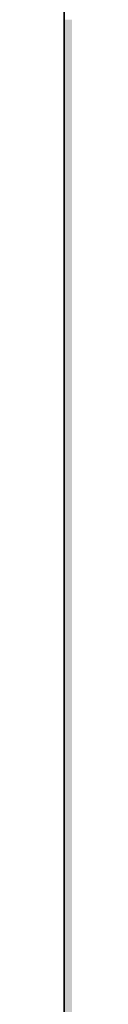
# Model space of a CAD drawing. Units: inches. Extents: x 2091 to 2899, y 967 to 2217.
# Tile 113 of 256: x 2203 to 2203, y 1131 to 1152. Entities that reach past the tile are written whole.
import ezdxf

# ---------------------------------------------------------------- set-up
doc = ezdxf.new("R2010")
doc.units = ezdxf.units.IN
doc.layers.add('A-WALL-PATT', color=141, linetype='Continuous', lineweight=13, true_color=0xadddf7)
doc.layers.add('C-PROP', color=7, linetype='Continuous', lineweight=35)

msp = doc.modelspace()

# ---------------------------------------------------------------- hatches: boundary and pattern name
at = {"layer": 'A-WALL-PATT'}
h = msp.add_hatch(color=256, dxfattribs=at)
h.dxf.hatch_style = 1
h.paths.add_polyline_path([(2212.144, 1941.419), (2387.644, 1941.419), (2387.644, 1824.419), (2392.144, 1824.419), (2392.144, 1941.419), (2609.644, 1941.419), (2609.644, 1825.919), (2614.144, 1825.919), (2614.144, 1941.419), (2794.144, 1941.419), (2794.144, 1928.762), (2803.144, 1928.762), (2803.144, 2050.919), (2203.144, 2050.919), (2203.144, 1900.758), (2212.144, 1900.758)])
h.paths.add_polyline_path([(2212.144, 1945.919), (2212.144, 2041.919), (2794.144, 2041.919), (2794.144, 1945.919), (2402.248, 1945.919), (2401.102, 1945.776), (2398.702, 1945.776)], flags=16)
h.paths.add_polyline_path([(2230.23, 1948.063), (2227.35, 1949.503), (2225.91, 1951.903), (2223.99, 1952.863), (2223.03, 1955.263), (2222.07, 1959.583), (2222.07, 1963.423), (2223.03, 1965.663), (2223.99, 1965.343), (2225.586, 1963.861), (2226.912, 1964.957), (2226.949, 1965.939), (2227.778, 1966.952), (2228.2, 1968.879), (2230.71, 1964.863), (2233.59, 1966.303), (2233.607, 1966.332), (2233.773, 1964.938), (2234.634, 1963.676), (2235.03, 1963.903), (2236.282, 1965.572), (2235.99, 1962.943), (2237.955, 1957.54), (2238.39, 1957.903), (2239.216, 1960.306), (2238.655, 1966.385), (2238.693, 1966.438), (2238.841, 1967.5), (2238.78, 1967.687), (2238.881, 1967.787), (2238.667, 1966.252), (2239.216, 1960.306), (2238.39, 1957.903), (2236.95, 1956.703), (2234.55, 1949.983)], flags=0)
h.paths.add_polyline_path([(2278.012, 1948.063), (2276.496, 1947.873), (2275.85, 1947.689), (2274.652, 1947.103)], flags=0)
h.paths.add_polyline_path([(2269.852, 1955.743), (2268.276, 1956.629), (2270.867, 1956.348), (2269.372, 1958.143), (2268.715, 1959.192), (2270.57, 1958.729), (2268.581, 1961.906), (2270.812, 1960.892), (2270.812, 1963.423), (2271.393, 1964.779), (2270.292, 1966.156), (2271.772, 1965.663), (2272.141, 1966.525), (2273.93, 1965.929), (2275.63, 1968.054), (2276.332, 1966.722), (2276.52, 1966.952), (2276.942, 1968.879), (2277.734, 1967.611), (2278.14, 1969.465), (2279.659, 1967.034), (2280.412, 1966.783), (2280.949, 1967.589), (2281.61, 1967.369), (2282.133, 1968.154), (2282.349, 1966.333), (2282.35, 1966.333), (2283.408, 1968.095), (2283.713, 1965.524), (2284.32, 1964.634), (2284.512, 1964.889), (2284.235, 1965.705), (2284.5, 1967.319), (2284.908, 1965.417), (2285.396, 1966.069), (2285.433, 1966.291), (2285.473, 1966.171), (2286.354, 1967.345), (2286.222, 1966.158), (2287.663, 1968.08), (2287.714, 1968.443), (2288.482, 1969.017), (2288.574, 1968.729), (2288.917, 1969.069), (2288.607, 1966.838), (2288.929, 1963.351), (2288.935, 1963.357), (2288.93, 1963.34), (2289.015, 1962.414), (2290.111, 1963.875), (2290.133, 1963.943), (2290.218, 1964.017), (2290.111, 1963.875), (2289.156, 1960.892), (2288.594, 1959.257), (2288.572, 1959.103), (2289.532, 1960.543), (2290.012, 1962.463), (2290.192, 1962.643), (2289.77, 1959.689), (2286.89, 1957.289), (2284.49, 1950.569), (2283.315, 1950.046), (2283.292, 1949.983), (2280.29, 1948.649), (2281.13, 1948.649), (2282.57, 1948.169), (2283.205, 1948.063), (2278.972, 1948.063), (2276.092, 1949.503), (2274.652, 1951.903), (2272.732, 1952.863)], flags=0)
h.paths.add_polyline_path([(2271.159, 1958.022), (2272.97, 1955.849), (2272.01, 1960.169), (2272.01, 1964.009), (2272.624, 1965.443), (2274.328, 1963.861), (2275.654, 1964.957), (2275.638, 1964.539), (2277.412, 1966.007), (2277.033, 1965.157), (2276.83, 1964.976), (2276.766, 1963.295), (2277.45, 1962.66), (2279.452, 1964.863), (2282.332, 1966.303), (2283.53, 1966.889), (2283.295, 1966.771), (2283.913, 1963.885), (2284.899, 1964.448), (2284.732, 1962.943), (2286.697, 1957.54), (2287.132, 1957.903), (2287.542, 1959.095), (2287.779, 1958.442), (2285.683, 1956.695), (2285.877, 1959.795), (2284.732, 1962.943), (2284.899, 1964.448), (2283.913, 1963.885), (2284.224, 1962.434), (2283.424, 1963.605), (2281.61, 1962.569), (2281.13, 1960.169), (2282.09, 1956.329), (2283.05, 1952.969), (2282.57, 1950.569), (2280.17, 1948.649), (2279.883, 1948.792), (2278.972, 1948.063), (2278.972, 1949.023), (2278.672, 1949.397), (2277.29, 1950.089), (2275.85, 1952.489), (2273.93, 1953.449), (2272.49, 1954.889), (2271.922, 1954.889), (2271.772, 1955.263)], flags=0)
h.paths.add_polyline_path([(2311.994, 1955.743), (2312.063, 1955.674), (2312.055, 1955.709)], flags=0)
h.paths.add_polyline_path([(2331.956, 1963.952), (2333.396, 1965.392), (2331.077, 1963.357), (2330.999, 1963.112)], flags=0)
h.paths.add_polyline_path([(2310.554, 1954.303), (2307.04, 1956.28), (2310.763, 1955.876), (2312.474, 1953.823), (2313.434, 1951.423), (2315.354, 1950.463), (2316.794, 1948.063), (2317.466, 1947.727), (2319.369, 1947.965), (2317.754, 1949.983), (2317.57, 1950.61), (2316.794, 1951.903), (2314.874, 1952.863), (2313.914, 1955.263), (2311.514, 1958.143), (2309.375, 1961.559), (2311.514, 1960.337), (2311.514, 1961.983), (2310.605, 1963.12), (2311.727, 1962.479), (2312.418, 1964.093), (2312.256, 1964.296), (2313.194, 1963.983), (2313.914, 1965.663), (2314.647, 1965.419), (2315.354, 1966.303), (2316.794, 1967.743), (2316.157, 1966.947), (2317.034, 1965.282), (2317.223, 1965.512), (2317.777, 1968.046), (2318.474, 1966.722), (2318.663, 1966.952), (2319.084, 1968.879), (2321.207, 1965.482), (2322.161, 1966.914), (2322.554, 1966.783), (2322.786, 1967.131), (2322.882, 1966.324), (2323.312, 1965.722), (2323.651, 1965.891), (2324.396, 1967.133), (2324.657, 1964.938), (2324.972, 1964.477), (2325.387, 1967.001), (2325.941, 1964.418), (2327.229, 1966.136), (2327.166, 1965.572), (2328.059, 1966.763), (2328.225, 1966.247), (2329.668, 1967.677), (2329.665, 1967.687), (2329.765, 1967.787), (2329.551, 1966.252), (2330.1, 1960.306), (2329.333, 1958.073), (2329.313, 1957.935), (2329.634, 1958.203), (2330.234, 1959.103), (2330.714, 1961.023), (2331.034, 1961.343), (2330.714, 1959.103), (2329.634, 1958.203), (2329.274, 1957.663), (2327.712, 1956.361), (2325.434, 1949.983), (2324.334, 1949.494), (2323.994, 1948.543), (2319.674, 1946.623), (2316.794, 1948.063), (2315.354, 1950.463), (2313.434, 1951.423)], flags=0)
h.paths.add_polyline_path([(2321.336, 1947.952), (2321.114, 1948.063), (2321.114, 1949.023), (2319.194, 1951.423), (2316.794, 1959.583), (2316.663, 1959.583), (2315.354, 1958.143), (2314.394, 1958.143), (2313.148, 1958.709), (2312.954, 1959.583), (2312.954, 1960.892), (2315.834, 1959.583), (2316.663, 1959.583), (2317.315, 1960.299), (2315.03, 1962.421), (2316.356, 1963.517), (2316.372, 1963.952), (2316.47, 1963.861), (2317.796, 1964.957), (2317.755, 1963.89), (2319.175, 1965.157), (2319.498, 1965.881), (2321.114, 1965.343), (2323.236, 1962.372), (2325.686, 1963.773), (2325.543, 1962.481), (2325.199, 1963.494), (2324.479, 1963.082), (2324.926, 1960.994), (2324.078, 1962.236), (2322.415, 1961.286), (2322.074, 1959.583), (2323.034, 1955.743), (2323.994, 1952.383), (2323.514, 1949.983), (2322.143, 1948.886), (2322.074, 1948.543)], flags=0)
h.paths.add_polyline_path([(2320.207, 1963.337), (2320.154, 1963.423), (2320.394, 1963.543)], flags=0)
h.paths.add_polyline_path([(2353.851, 1965.811), (2354.031, 1965.751), (2354.331, 1966.451), (2354.331, 1966.931)], flags=0)
h.paths.add_polyline_path([(2359.021, 1969.026), (2359.098, 1968.902), (2359.234, 1969.52), (2359.234, 1970)], flags=0)
h.paths.add_polyline_path([(2358.257, 1966.682), (2357.984, 1966.348), (2358.211, 1966.146), (2358.41, 1966.39)], flags=0)
h.paths.add_polyline_path([(2357.768, 1966.059), (2357.732, 1965.105), (2357.751, 1965.121), (2357.77, 1965.607), (2357.77, 1966.058)], flags=0)
h.paths.add_polyline_path([(2359.112, 1965.305), (2359.112, 1964.825), (2359.845, 1966.468), (2359.845, 1966.948)], flags=0)
h.paths.add_polyline_path([(2360.224, 1966.621), (2360.699, 1969.363), (2360.699, 1969.843), (2360.211, 1967.026), (2360.211, 1966.643)], flags=0)
h.paths.add_polyline_path([(2363.451, 1967.891), (2363.451, 1968.371), (2362.491, 1966.931), (2362.656, 1966.699)], flags=0)
h.paths.add_polyline_path([(2364.476, 1966.079), (2365.851, 1968.371), (2365.851, 1968.851), (2364.428, 1966.48)], flags=0)
h.paths.add_polyline_path([(2366.314, 1965.853), (2366.367, 1965.696), (2366.803, 1968.346), (2366.803, 1968.826)], flags=0)
h.paths.add_polyline_path([(2367.165, 1965.804), (2367.291, 1966.931), (2367.291, 1967.411), (2367.103, 1965.72)], flags=0)
h.paths.add_polyline_path([(2370.037, 1959.974), (2371.014, 1963.025), (2371.014, 1963.505), (2370.037, 1960.454)], flags=0)
h.paths.add_polyline_path([(2371.611, 1960.211), (2372.571, 1961.651), (2372.571, 1962.131), (2371.803, 1960.979)], flags=0)
h.paths.add_polyline_path([(2350.874, 1956.005), (2351.931, 1955.891), (2354.491, 1953.331), (2353.851, 1954.931), (2351.451, 1957.811), (2347.936, 1963.426), (2347.936, 1963.906), (2351.451, 1958.291), (2353.705, 1955.585), (2352.891, 1959.251), (2352.891, 1959.731), (2352.891, 1961.925), (2356.731, 1959.731), (2358.454, 1961.627), (2354.811, 1965.011), (2355.031, 1965.286), (2358.691, 1961.887), (2361.531, 1965.011), (2364.376, 1966.433), (2364.524, 1965.187), (2365.454, 1963.824), (2365.881, 1964.068), (2365.371, 1966.451), (2365.371, 1966.931), (2366.811, 1960.211), (2366.811, 1959.731), (2366.389, 1952.981), (2367.771, 1956.851), (2368.641, 1957.576), (2366.811, 1962.611), (2366.811, 1963.091), (2368.775, 1957.688), (2369.211, 1958.051), (2370.002, 1960.352), (2369.475, 1966.053), (2369.513, 1966.106), (2369.514, 1966.111), (2369.475, 1966.533), (2369.513, 1966.586), (2369.615, 1967.313), (2369.183, 1968.659), (2369.183, 1969.139), (2369.601, 1967.835), (2369.701, 1967.934), (2369.718, 1968.055), (2370.145, 1968.374), (2369.779, 1968.011), (2369.701, 1967.454), (2370.468, 1968.214), (2369.675, 1967.266), (2369.514, 1966.111), (2370.037, 1960.454), (2370.037, 1959.974), (2369.442, 1958.243), (2370.651, 1959.251), (2371.046, 1962.018), (2371.131, 1962.131), (2370.651, 1958.771), (2367.771, 1956.371), (2365.371, 1949.651), (2362.079, 1948.188), (2363.451, 1947.731), (2361.051, 1947.731), (2360.091, 1947.731), (2357.104, 1947.357), (2360.091, 1948.211), (2358.171, 1949.171), (2356.731, 1951.571), (2354.811, 1952.531), (2351.931, 1955.411)], flags=0)
h.paths.add_polyline_path([(2361.051, 1948.691), (2359.131, 1951.091), (2356.731, 1959.251), (2355.771, 1959.251), (2352.891, 1960.56), (2352.891, 1961.445), (2355.891, 1959.731), (2356.731, 1959.731), (2356.837, 1959.368), (2361.531, 1964.531), (2363.248, 1965.389), (2364.925, 1963.042), (2362.491, 1961.651), (2362.064, 1959.517), (2362.971, 1955.891), (2363.931, 1952.531), (2363.931, 1952.051), (2363.451, 1949.651), (2361.051, 1947.731)], flags=0)
h.paths.add_polyline_path([(2359.131, 1951.571), (2359.291, 1951.371), (2361.051, 1954.451), (2361.051, 1954.931)], flags=0)
h.paths.add_polyline_path([(2357.22, 1966.546), (2356.793, 1968.815), (2356.793, 1969.295), (2357.22, 1967.026)], flags=0)
h.paths.add_polyline_path([(2361.051, 1954.451), (2361.531, 1958.771), (2361.531, 1959.251), (2361.051, 1954.931)], flags=0)
h.paths.add_polyline_path([(2402.548, 1948.486), (2402.302, 1948.416), (2402.59, 1948.416)], flags=0)
h.paths.add_polyline_path([(2394.142, 1956.096), (2395.685, 1954.553), (2396.72, 1953.971), (2396.062, 1955.616), (2395.241, 1956.601), (2395.879, 1956.442), (2395.102, 1959.936), (2395.102, 1963.776), (2396.062, 1966.016), (2397.022, 1965.696), (2398.618, 1964.214), (2399.944, 1965.31), (2399.981, 1966.292), (2400.811, 1967.305), (2401.232, 1969.232), (2403.538, 1965.543), (2403.942, 1967.389), (2404.702, 1967.136), (2405.46, 1966.075), (2406.622, 1966.656), (2406.64, 1966.685), (2406.805, 1965.291), (2406.926, 1965.115), (2407.342, 1964.976), (2407.874, 1965.774), (2408.169, 1964.398), (2409.315, 1965.925), (2409.217, 1965.051), (2409.445, 1963.131), (2410.306, 1961.87), (2410.702, 1962.096), (2411.442, 1963.082), (2411.165, 1963.898), (2411.616, 1966.64), (2411.725, 1966.791), (2411.873, 1967.853), (2411.813, 1968.041), (2411.913, 1968.14), (2411.699, 1966.605), (2412.248, 1960.659), (2413.225, 1963.71), (2414.378, 1964.721), (2414.513, 1965.693), (2414.453, 1965.881), (2414.553, 1965.98), (2414.378, 1964.721), (2414.52, 1964.846), (2414.365, 1964.631), (2414.339, 1964.445), (2414.888, 1958.499), (2414.062, 1956.096), (2412.622, 1954.896), (2410.171, 1948.033), (2410.017, 1948.084), (2405.902, 1946.256), (2405.902, 1947.216), (2405.204, 1948.089), (2404.222, 1948.416), (2403.262, 1948.416), (2400.382, 1949.856), (2399.662, 1951.056), (2397.982, 1952.736), (2397.022, 1953.216), (2395.685, 1954.553), (2392.657, 1956.257)], flags=0)
h.paths.add_polyline_path([(2409.086, 1964.407), (2409.13, 1964.276), (2409.262, 1964.496)], flags=0)
h.paths.add_polyline_path([(2397.742, 1961.616), (2398.702, 1963.856), (2399.662, 1963.536), (2401.427, 1965.741), (2401.791, 1966.559), (2402.071, 1965.071), (2402.836, 1964.393), (2403.262, 1964.915), (2403.338, 1964.771), (2402.616, 1963.976), (2402.499, 1960.902), (2403.543, 1959.932), (2404.413, 1960.89), (2404.702, 1962.336), (2407.916, 1964.172), (2409.52, 1961.927), (2410.987, 1957.893), (2411.422, 1958.256), (2412.048, 1960.076), (2412.41, 1959.079), (2411.676, 1958.467), (2411.662, 1958.256), (2411.626, 1958.426), (2409.982, 1957.056), (2407.582, 1950.336), (2403.262, 1948.416), (2403.262, 1949.376), (2401.342, 1951.776), (2399.417, 1958.324), (2397.742, 1959.085), (2397.742, 1959.97), (2397.102, 1960.336), (2397.742, 1960.045)], flags=0)
h.paths.add_polyline_path([(2405.902, 1952.976), (2405.95, 1953.408), (2406.017, 1953.176)], flags=0)
h.paths.add_polyline_path([(2449.818, 1967.114), (2449.752, 1967.136), (2449.794, 1967.078)], flags=0)
h.paths.add_polyline_path([(2451.698, 1966.618), (2451.741, 1966.69), (2451.692, 1966.666)], flags=0)
h.paths.add_polyline_path([(2454.344, 1965.738), (2455.752, 1967.616), (2455.992, 1968.096), (2454.364, 1965.925)], flags=0)
h.paths.add_polyline_path([(2457.547, 1968.864), (2457.787, 1969.344), (2457.054, 1968.796), (2457.008, 1968.46)], flags=0)
h.paths.add_polyline_path([(2456.922, 1967.857), (2456.802, 1968.229), (2456.723, 1967.66)], flags=0)
h.paths.add_polyline_path([(2457.302, 1967.377), (2457.542, 1967.857), (2456.81, 1966.84), (2456.741, 1966.7), (2456.749, 1966.608)], flags=0)
h.paths.add_polyline_path([(2458.275, 1963.71), (2458.155, 1963.335), (2460.354, 1965.265), (2460.594, 1965.745)], flags=0)
h.paths.add_polyline_path([(2458.392, 1962.816), (2458.364, 1962.618), (2459.592, 1964.256), (2459.832, 1964.736)], flags=0)
h.paths.add_polyline_path([(2459.352, 1962.816), (2459.272, 1962.496), (2460.072, 1963.296), (2460.312, 1963.776)], flags=0)
h.paths.add_polyline_path([(2458.68, 1960.608), (2458.632, 1960.416), (2459.592, 1961.856), (2459.832, 1962.336)], flags=0)
h.paths.add_polyline_path([(2437.838, 1956.243), (2439.192, 1956.096), (2441.352, 1953.936), (2440.872, 1955.136), (2438.472, 1958.016), (2438.072, 1958.656), (2438.712, 1958.496), (2440.64, 1956.183), (2439.912, 1959.456), (2439.912, 1963.296), (2441.352, 1966.656), (2441.592, 1967.136), (2441.112, 1966.016), (2442.072, 1965.696), (2443.989, 1968.092), (2444.241, 1966.751), (2444.917, 1966.152), (2445.677, 1967.08), (2446.255, 1969.725), (2446.495, 1970.205), (2446.282, 1969.232), (2447.363, 1967.503), (2447.72, 1969.568), (2447.96, 1970.048), (2447.485, 1967.307), (2448.792, 1965.216), (2448.472, 1964.864), (2448.552, 1964.736), (2451.452, 1966.186), (2451.615, 1964.811), (2452.308, 1963.796), (2453.235, 1964.326), (2454.072, 1960.416), (2453.629, 1953.318), (2454.792, 1956.576), (2455.032, 1957.056), (2455.719, 1957.628), (2453.832, 1962.816), (2453.941, 1963.794), (2453.335, 1965.578), (2453.824, 1968.551), (2454.064, 1969.031), (2453.575, 1966.058), (2454.04, 1964.688), (2453.832, 1962.816), (2455.719, 1957.628), (2456.367, 1958.168), (2457.058, 1960.179), (2457.298, 1960.659), (2456.472, 1958.256), (2457.718, 1959.294), (2457.672, 1958.976), (2454.89, 1956.657), (2453.614, 1953.085), (2453.592, 1952.736), (2453.352, 1952.256), (2453.36, 1952.372), (2452.632, 1950.336), (2452.392, 1949.856), (2449.204, 1948.439), (2450.712, 1947.936), (2448.072, 1947.936), (2447.112, 1947.936), (2444.552, 1947.616), (2447.2, 1948.372), (2445.192, 1949.376), (2443.752, 1951.776), (2441.832, 1952.736), (2438.952, 1955.616)], flags=0)
h.paths.add_polyline_path([(2443.992, 1959.936), (2444.04, 1959.773), (2444.122, 1959.862)], flags=0)
h.paths.add_polyline_path([(2442.912, 1959.936), (2443.032, 1959.936), (2442.446, 1960.202)], flags=0)
h.paths.add_polyline_path([(2444.983, 1965.02), (2445.279, 1965.265), (2445.519, 1965.745), (2444.994, 1965.31)], flags=0)
h.paths.add_polyline_path([(2446.133, 1965.03), (2446.33, 1965.471), (2444.97, 1964.258), (2444.73, 1963.778)], flags=0)
h.paths.add_polyline_path([(2442.792, 1959.456), (2443.752, 1959.456), (2446.152, 1951.296), (2446.412, 1951.751), (2446.392, 1951.776), (2448.081, 1954.73), (2448.552, 1958.976), (2441.832, 1965.216), (2442.155, 1965.619), (2448.792, 1959.456), (2448.312, 1955.136), (2448.072, 1954.656), (2446.412, 1951.751), (2448.312, 1949.376), (2448.312, 1948.416), (2450.541, 1950.199), (2450.952, 1952.256), (2449.992, 1955.616), (2449.032, 1959.456), (2449.512, 1961.856), (2449.752, 1962.336), (2449.675, 1961.949), (2452.995, 1963.846), (2453.064, 1963.519), (2452.885, 1963.783), (2449.675, 1961.949), (2449.272, 1959.936), (2450.232, 1956.096), (2451.192, 1952.736), (2450.712, 1950.336), (2450.472, 1949.856), (2448.072, 1947.936), (2448.072, 1948.536), (2445.432, 1949.856), (2443.992, 1952.256), (2442.072, 1953.216), (2441.112, 1955.616), (2440.152, 1959.936), (2440.152, 1960.656)], flags=0)
h.paths.add_polyline_path([(2456.692, 1966.986), (2457.608, 1968.081), (2457.848, 1968.561), (2456.932, 1967.466)], flags=0)
h.paths.add_polyline_path([(2489.897, 1966.58), (2489.943, 1966.189), (2490.747, 1967.53), (2491.319, 1968.951)], flags=0)
h.paths.add_polyline_path([(2473.562, 1956.407), (2477.14, 1956.019), (2476.955, 1956.241), (2475.108, 1957.28), (2476.347, 1956.97), (2475.187, 1958.824), (2476.919, 1958.391), (2475.412, 1960.799), (2477.787, 1959.719), (2477.787, 1962.25), (2477.637, 1962.438), (2477.823, 1962.332), (2478.359, 1963.584), (2478.359, 1963.671), (2477.324, 1964.965), (2478.715, 1964.501), (2479.319, 1965.911), (2480.279, 1965.591), (2481.784, 1967.472), (2482.116, 1965.705), (2482.881, 1965.028), (2483.209, 1965.429), (2483.22, 1965.715), (2483.076, 1965.989), (2483.712, 1966.766), (2484.13, 1968.679), (2484.702, 1970.1), (2484.489, 1969.127), (2486.503, 1965.905), (2487.387, 1965.61), (2488.153, 1966.759), (2488.717, 1965.97), (2489.2, 1966.212), (2489.331, 1965.111), (2490.394, 1963.622), (2490.661, 1963.775), (2490.494, 1964.554), (2490.923, 1963.925), (2491.319, 1964.151), (2491.333, 1964.17), (2491.21, 1964.532), (2491.282, 1964.966), (2491.426, 1964.293), (2494.076, 1967.828), (2494.498, 1966.515), (2494.598, 1966.614), (2494.689, 1967.27), (2495.107, 1967.582), (2495.13, 1967.748), (2495.07, 1967.936), (2495.17, 1968.035), (2495.032, 1967.044), (2495.754, 1967.759), (2494.982, 1966.686), (2494.956, 1966.5), (2495.479, 1960.837), (2495.91, 1962.184), (2496.482, 1963.605), (2496.073, 1962.327), (2496.769, 1962.938), (2496.599, 1962.711), (2496.119, 1959.351), (2496.733, 1960.272), (2496.987, 1961.29), (2497.559, 1962.711), (2497.079, 1960.791), (2496.507, 1959.37), (2495.547, 1957.93), (2492.759, 1955.606), (2490.839, 1950.231), (2490.267, 1948.81), (2485.947, 1946.89), (2483.067, 1948.33), (2481.627, 1950.73), (2479.707, 1951.69), (2476.827, 1954.57)], flags=0)
h.paths.add_polyline_path([(2485.577, 1948.313), (2485.559, 1948.311), (2485.579, 1948.311)], flags=0)
h.paths.add_polyline_path([(2478.645, 1954.551), (2478.109, 1956.963), (2479.319, 1955.511), (2480.279, 1953.111), (2482.199, 1952.151), (2483.639, 1949.751), (2486.519, 1948.311), (2486.519, 1949.271), (2484.739, 1951.496), (2484.027, 1950.25), (2481.627, 1958.41), (2482.375, 1959.233), (2482.199, 1959.831), (2483.198, 1960.929), (2479.707, 1964.17), (2480.603, 1965.29), (2481.875, 1964.109), (2482.666, 1964.764), (2482.615, 1963.422), (2482.989, 1963.075), (2484.008, 1963.984), (2484.684, 1965.498), (2484.58, 1965.405), (2485.357, 1967.147), (2485.121, 1965.781), (2486.427, 1963.69), (2488.145, 1964.549), (2489.822, 1962.202), (2490.747, 1962.73), (2492, 1964.4), (2492.076, 1965.087), (2492.213, 1964.684), (2492.485, 1965.047), (2492.279, 1963.191), (2494.244, 1957.788), (2494.563, 1958.054), (2494.933, 1959.133), (2495.505, 1960.554), (2494.679, 1958.151), (2494.107, 1956.73), (2494.563, 1958.054), (2493.409, 1957.092), (2491.707, 1961.77), (2492, 1964.4), (2490.747, 1962.73), (2487.712, 1960.996), (2487.479, 1959.831), (2488.439, 1955.991), (2489.399, 1952.631), (2488.919, 1950.231), (2488.577, 1949.957), (2488.347, 1948.81), (2487.652, 1948.254), (2487.479, 1948.311), (2486.519, 1948.311), (2483.639, 1949.751), (2482.199, 1952.151), (2480.279, 1953.111), (2478.839, 1954.551)], flags=0)
h.paths.add_polyline_path([(2526.648, 1966.988), (2526.517, 1967.031), (2526.6, 1966.915)], flags=0)
h.paths.add_polyline_path([(2528.471, 1966.447), (2528.574, 1966.62), (2528.457, 1966.561)], flags=0)
h.paths.add_polyline_path([(2534.133, 1967.496), (2534.157, 1967.543), (2534.06, 1967.408)], flags=0)
h.paths.add_polyline_path([(2536.162, 1964.051), (2535.157, 1962.711), (2535.101, 1962.316), (2536.117, 1963.671), (2536.421, 1964.278)], flags=0)
h.paths.add_polyline_path([(2535.157, 1959.831), (2536.117, 1961.271), (2536.597, 1962.231), (2535.253, 1960.215)], flags=0)
h.paths.add_polyline_path([(2513.249, 1956.285), (2516.221, 1955.963), (2514.997, 1957.431), (2514.196, 1958.712), (2515.477, 1958.391), (2516.932, 1956.646), (2516.437, 1958.871), (2516.437, 1962.711), (2516.873, 1963.727), (2515.346, 1965.635), (2517.397, 1964.951), (2517.877, 1966.071), (2518.357, 1967.031), (2517.877, 1965.911), (2518.837, 1965.591), (2520.487, 1967.653), (2520.766, 1966.166), (2521.53, 1965.489), (2521.781, 1965.795), (2521.801, 1966.307), (2521.478, 1966.921), (2521.246, 1967.126), (2521.178, 1967.491), (2521.478, 1966.921), (2522.01, 1966.449), (2522.257, 1966.75), (2522.78, 1969.14), (2523.26, 1970.1), (2523.047, 1969.127), (2524.673, 1966.526), (2526.037, 1966.071), (2526.795, 1965.01), (2527.977, 1965.601), (2528.14, 1964.227), (2528.665, 1963.458), (2529.389, 1963.872), (2529.33, 1964.147), (2529.481, 1963.925), (2529.877, 1964.151), (2529.984, 1964.293), (2529.789, 1965.203), (2530.062, 1964.398), (2532.802, 1968.051), (2533.148, 1966.976), (2533.248, 1967.075), (2533.339, 1967.731), (2533.673, 1967.98), (2533.728, 1968.035), (2533.514, 1966.5), (2534.025, 1960.972), (2534.56, 1962.645), (2535.04, 1963.605), (2534.063, 1960.554), (2533.237, 1958.151), (2534.288, 1959.027), (2534.197, 1958.391), (2531.513, 1956.154), (2529.397, 1950.231), (2528.917, 1949.271), (2526.449, 1948.174), (2527.477, 1947.831), (2530.357, 1947.351), (2524.597, 1947.351), (2521.717, 1948.791), (2520.277, 1951.191), (2518.357, 1952.151), (2515.477, 1955.031)], flags=0)
h.paths.add_polyline_path([(2523.935, 1967.19), (2523.62, 1966.484), (2523.77, 1966.242)], flags=0)
h.paths.add_polyline_path([(2518.837, 1953.111), (2517.877, 1955.511), (2516.885, 1959.977), (2516.917, 1959.962), (2516.917, 1962.025), (2520.757, 1959.831), (2522.025, 1961.226), (2518.357, 1964.631), (2519.003, 1965.438), (2520.433, 1964.109), (2521.301, 1964.827), (2521.245, 1963.355), (2525.638, 1959.276), (2526.037, 1961.271), (2529.397, 1963.191), (2530.65, 1964.861), (2530.665, 1964.998), (2530.692, 1964.917), (2531.088, 1965.445), (2530.946, 1964.169), (2530.692, 1964.917), (2529.397, 1963.191), (2526.363, 1961.457), (2526.037, 1959.831), (2526.997, 1955.991), (2527.957, 1952.631), (2527.477, 1950.231), (2527.134, 1949.957), (2526.974, 1949.154), (2526.697, 1949.031), (2524.597, 1947.351), (2524.597, 1948.311), (2524.277, 1948.711), (2522.197, 1949.751), (2520.757, 1952.151)], flags=0)
h.paths.add_polyline_path([(2520.277, 1958.871), (2520.853, 1959.505), (2523.157, 1951.671), (2524.614, 1954.22), (2524.597, 1954.071), (2522.677, 1950.711)], flags=0)
h.paths.add_polyline_path([(2559.371, 1966.311), (2559.398, 1966.325), (2559.402, 1966.345)], flags=0)
h.paths.add_polyline_path([(2549.771, 1957.191), (2552.651, 1954.311), (2552.134, 1955.603), (2550.611, 1957.431), (2547.096, 1963.046), (2545.776, 1965.206), (2549.291, 1959.591), (2551.691, 1956.711), (2550.793, 1960.752), (2550.731, 1960.78), (2550.731, 1964.871), (2551.691, 1967.111), (2552.651, 1966.791), (2554.247, 1965.309), (2555.034, 1965.96), (2555.582, 1966.645), (2555.61, 1967.387), (2556.439, 1968.401), (2556.861, 1970.327), (2559.371, 1966.311), (2560.691, 1964.151), (2562.409, 1965.01), (2561.651, 1966.071), (2560.331, 1968.231), (2561.758, 1966.233), (2562.347, 1967.116), (2562.434, 1966.387), (2563.128, 1965.37), (2563.571, 1965.591), (2563.588, 1965.62), (2563.363, 1967.524), (2563.722, 1965.844), (2565.06, 1968.073), (2564.733, 1965.129), (2565.118, 1963.333), (2567.445, 1966.436), (2567.316, 1967.833), (2567.354, 1967.886), (2567.502, 1968.948), (2567.441, 1969.136), (2567.542, 1969.235), (2567.328, 1967.7), (2567.877, 1961.754), (2568.747, 1964.47), (2568.636, 1965.673), (2568.674, 1965.726), (2568.822, 1966.788), (2568.761, 1966.976), (2568.862, 1967.075), (2568.648, 1965.54), (2568.726, 1964.693), (2568.854, 1964.805), (2568.747, 1964.47), (2568.817, 1963.706), (2568.971, 1963.911), (2568.866, 1963.177), (2569.197, 1959.594), (2568.371, 1957.191), (2566.931, 1955.991), (2564.62, 1949.521), (2564.651, 1949.511), (2564.617, 1949.511), (2564.531, 1949.271), (2560.211, 1947.351), (2557.331, 1948.791), (2556.045, 1950.934), (2556.011, 1950.951), (2555.857, 1951.208), (2553.971, 1952.151), (2551.091, 1955.031), (2546.65, 1957.53)], flags=0)
h.paths.add_polyline_path([(2567.026, 1959.33), (2567.035, 1959.305), (2567.051, 1959.351)], flags=0)
h.paths.add_polyline_path([(2551.968, 1962.518), (2553.011, 1964.951), (2553.971, 1964.631), (2555.567, 1963.149), (2556.893, 1964.246), (2556.93, 1965.227), (2557.144, 1965.489), (2556.42, 1966.131), (2556.391, 1966.105), (2556.38, 1966.166), (2556.42, 1966.131), (2556.952, 1966.605), (2557.092, 1966.919), (2557.571, 1966.01), (2557.759, 1966.241), (2557.418, 1964.68), (2556.893, 1964.246), (2556.807, 1961.998), (2560.691, 1958.391), (2560.636, 1957.893), (2560.811, 1957.191), (2561.771, 1953.831), (2561.291, 1951.431), (2559.11, 1949.687), (2559.156, 1949.629), (2563.027, 1951.349), (2562.611, 1949.271), (2560.211, 1947.351), (2560.211, 1948.311), (2559.251, 1949.511), (2558.891, 1949.511), (2558.891, 1949.961), (2558.291, 1950.711), (2558.054, 1951.518), (2556.971, 1952.871), (2555.068, 1959.341), (2552.051, 1961.065), (2552.051, 1962.471)], flags=0)
h.paths.add_polyline_path([(2588.33, 1958.391), (2588.61, 1958.111), (2588.553, 1958.367)], flags=0)
h.paths.add_polyline_path([(2594.745, 1950.493), (2593.958, 1953.172), (2593.13, 1954.551), (2591.21, 1955.511), (2590.25, 1957.911), (2588.309, 1960.24), (2586.177, 1961.209), (2587.85, 1960.791), (2587.253, 1961.744), (2588.441, 1961.065), (2588.441, 1962.656), (2588.422, 1962.665), (2588.441, 1962.711), (2586.914, 1964.62), (2588.877, 1963.728), (2589.29, 1964.692), (2589.29, 1966.071), (2590.25, 1968.311), (2591.21, 1967.991), (2592.806, 1966.509), (2594.132, 1967.606), (2594.169, 1968.587), (2594.999, 1969.601), (2595.42, 1971.527), (2597.93, 1967.511), (2600.81, 1968.951), (2600.827, 1968.98), (2600.993, 1967.587), (2601.854, 1966.325), (2602.107, 1966.47), (2602.236, 1967.255), (2602.357, 1966.693), (2603.502, 1968.221), (2603.21, 1965.591), (2605.175, 1960.188), (2605.507, 1960.465), (2605.026, 1965.673), (2605.064, 1965.726), (2605.212, 1966.788), (2605.152, 1966.976), (2605.252, 1967.075), (2605.343, 1967.731), (2605.953, 1968.187), (2605.875, 1969.033), (2605.913, 1969.086), (2606.061, 1970.148), (2606, 1970.336), (2606.101, 1970.435), (2605.887, 1968.9), (2606.436, 1962.954), (2605.61, 1960.551), (2605.997, 1960.874), (2606.564, 1962.645), (2608.241, 1964.117), (2608.01, 1963.191), (2607.05, 1961.751), (2606.631, 1961.402), (2606.201, 1958.391), (2603.321, 1955.991), (2600.921, 1949.271), (2596.601, 1947.351), (2593.721, 1948.791), (2592.857, 1950.231), (2592.65, 1950.231)], flags=0)
h.paths.add_polyline_path([(2596.601, 1947.351), (2596.601, 1948.311), (2594.681, 1950.711), (2596.155, 1953.29), (2595.53, 1954.071), (2593.199, 1961.996), (2592.651, 1962.505), (2591.78, 1963.003), (2593.283, 1964.246), (2593.32, 1965.227), (2594.15, 1966.241), (2594.571, 1968.167), (2596.183, 1965.589), (2596.951, 1966.435), (2598.041, 1966.071), (2598.799, 1965.01), (2599.961, 1965.591), (2599.979, 1965.62), (2600.144, 1964.227), (2601.005, 1962.965), (2601.401, 1963.191), (2602.653, 1964.861), (2602.361, 1962.231), (2603.793, 1958.295), (2601.978, 1953.212), (2601.946, 1952.709), (2599.469, 1951.608), (2599.001, 1949.271)], flags=0)
h.paths.add_polyline_path([(2597.561, 1958.871), (2597.671, 1959.419), (2597.595, 1958.736)], flags=0)
h.paths.add_polyline_path([(2623.666, 1961.254), (2625.519, 1960.791), (2624.966, 1961.676), (2627.199, 1960.66), (2627.199, 1961.151), (2626.959, 1962.231), (2626.959, 1963.491), (2625.582, 1965.212), (2626.959, 1964.425), (2626.959, 1965.831), (2626.869, 1965.861), (2627.919, 1968.311), (2628.879, 1967.991), (2630.475, 1966.509), (2631.801, 1967.606), (2631.838, 1968.587), (2632.668, 1969.601), (2633.089, 1971.527), (2635.599, 1967.511), (2638.479, 1968.951), (2638.497, 1968.98), (2638.662, 1967.587), (2639.176, 1966.833), (2639.78, 1967.84), (2640.026, 1966.693), (2641.171, 1968.221), (2640.879, 1965.591), (2641.114, 1964.945), (2641.411, 1965.341), (2641.308, 1964.412), (2642.844, 1960.188), (2643.279, 1960.551), (2644.085, 1962.895), (2643.784, 1966.153), (2643.807, 1966.185), (2643.601, 1968.418), (2643.523, 1968.661), (2643.73, 1970.148), (2643.67, 1970.336), (2643.77, 1970.435), (2643.556, 1968.9), (2643.601, 1968.418), (2643.91, 1967.456), (2644.01, 1967.555), (2643.812, 1966.132), (2644.105, 1962.954), (2644.239, 1961.351), (2644.719, 1961.751), (2645.033, 1962.222), (2645.322, 1963.125), (2646.076, 1963.787), (2645.033, 1962.222), (2644.345, 1960.074), (2643.519, 1957.671), (2642.079, 1956.471), (2639.72, 1949.864), (2639.876, 1949.838), (2635.359, 1947.831), (2632.479, 1949.271), (2631.039, 1951.671), (2629.119, 1952.631), (2628.159, 1955.031), (2625.759, 1957.911)], flags=0)
h.paths.add_polyline_path([(2627.816, 1956.574), (2627.374, 1958.566), (2626.376, 1959.763), (2627.199, 1959.351), (2627.374, 1958.566), (2627.919, 1957.911), (2628.879, 1955.511), (2630.799, 1954.551), (2632.239, 1952.151), (2633.315, 1951.613), (2631.039, 1959.351), (2631.498, 1959.856), (2630.799, 1962.231), (2631.45, 1962.947), (2630.715, 1963.629), (2632.041, 1964.726), (2632.078, 1965.707), (2632.292, 1965.969), (2631.705, 1966.489), (2633.136, 1967.766), (2633.329, 1968.647), (2634.675, 1966.494), (2635.208, 1967.081), (2636.799, 1966.551), (2637.676, 1967.867), (2638.994, 1966.022), (2639.705, 1966.429), (2641.119, 1959.831), (2640.93, 1956.806), (2639.439, 1952.631), (2638.227, 1952.093), (2637.759, 1949.751), (2635.359, 1947.831), (2635.359, 1948.791), (2633.439, 1951.191), (2633.315, 1951.613), (2632.239, 1952.151), (2630.799, 1954.551), (2628.879, 1955.511)], flags=0)
h.paths.add_polyline_path([(2637.759, 1953.831), (2637.279, 1955.511), (2636.319, 1959.351), (2636.799, 1961.751), (2639.234, 1963.142), (2637.557, 1965.49), (2638.739, 1966.081), (2638.902, 1964.707), (2639.763, 1963.445), (2636.799, 1961.751), (2636.532, 1960.418), (2637.039, 1958.391), (2637.999, 1955.031)], flags=0)
h.paths.add_polyline_path([(2668.567, 1951.431), (2667.607, 1953.831), (2665.207, 1956.711), (2662.294, 1961.365), (2665.447, 1959.591), (2666.647, 1958.391), (2666.647, 1959.975), (2666.058, 1960.682), (2666.647, 1960.345), (2666.647, 1961.991), (2666.7, 1962.114), (2666.407, 1963.431), (2666.407, 1967.271), (2667.367, 1969.511), (2668.327, 1969.191), (2669.923, 1967.709), (2671.249, 1968.806), (2671.286, 1969.787), (2672.116, 1970.801), (2672.537, 1972.727), (2675.047, 1968.711), (2677.927, 1970.151), (2677.945, 1970.18), (2678.11, 1968.787), (2678.971, 1967.525), (2679.367, 1967.751), (2680.62, 1969.421), (2680.327, 1966.791), (2682.292, 1961.388), (2682.727, 1961.751), (2683.358, 1963.587), (2683.232, 1964.953), (2683.27, 1965.006), (2683.393, 1965.889), (2683.36, 1966.249), (2683.358, 1966.256), (2683.359, 1966.257), (2682.992, 1970.233), (2683.03, 1970.286), (2683.178, 1971.348), (2683.118, 1971.536), (2683.218, 1971.635), (2683.004, 1970.1), (2683.359, 1966.257), (2683.458, 1966.355), (2683.393, 1965.889), (2683.414, 1965.665), (2684.424, 1966.872), (2683.553, 1964.154), (2683.358, 1963.587), (2683.793, 1958.874), (2682.967, 1956.471), (2681.527, 1955.271), (2680.109, 1951.3), (2680.085, 1950.912), (2679.977, 1950.93), (2679.127, 1948.551), (2674.807, 1946.631), (2671.927, 1948.071), (2670.487, 1950.471)], flags=0)
h.paths.add_polyline_path([(2671.936, 1953.227), (2671.687, 1953.351), (2670.247, 1955.751), (2668.327, 1956.711), (2667.357, 1959.138), (2669.527, 1958.151), (2670.487, 1958.151), (2671.479, 1959.242), (2670.684, 1961.945), (2668.89, 1963.612), (2667.307, 1964.331), (2668.567, 1963.911), (2668.831, 1964.241), (2670.247, 1963.431), (2672.422, 1965.823), (2672.777, 1967.447), (2673.234, 1966.716), (2674.412, 1968.012), (2673.981, 1965.522), (2675.287, 1963.431), (2675.554, 1963.564), (2675.932, 1965.456), (2676.247, 1965.351), (2677.005, 1964.29), (2678.167, 1964.871), (2679.607, 1967.271), (2680.327, 1963.911), (2680.307, 1963.577), (2680.347, 1963.458), (2680.86, 1964.141), (2680.567, 1961.511), (2681.104, 1960.037), (2678.887, 1953.831), (2677.092, 1953.033), (2677.687, 1950.951), (2677.207, 1948.551), (2674.807, 1946.631), (2674.807, 1947.591), (2672.887, 1949.991)], flags=0)
h.paths.add_polyline_path([(2673.985, 1951.911), (2674.567, 1952.931), (2674.567, 1951.911), (2676.967, 1953.831), (2677.447, 1956.231), (2676.487, 1959.591), (2676.247, 1960.551), (2679.73, 1962.541), (2680.059, 1961.002), (2679.211, 1962.245), (2676.247, 1960.551), (2676.487, 1959.591), (2677.447, 1956.231), (2676.967, 1953.831), (2674.567, 1951.911)], flags=0)
h.paths.add_polyline_path([(2707.479, 1952.815), (2706.519, 1955.215), (2705.559, 1959.535), (2705.559, 1963.375), (2706.519, 1965.615), (2707.479, 1965.295), (2709.075, 1963.813), (2710.401, 1964.909), (2710.438, 1965.891), (2711.268, 1966.904), (2711.689, 1968.831), (2714.199, 1964.815), (2717.079, 1966.255), (2717.097, 1966.284), (2717.262, 1964.89), (2718.123, 1963.628), (2718.519, 1963.855), (2719.771, 1965.524), (2719.479, 1962.895), (2721.444, 1957.492), (2721.879, 1957.855), (2722.705, 1960.258), (2722.144, 1966.337), (2722.182, 1966.39), (2722.33, 1967.452), (2722.27, 1967.639), (2722.37, 1967.739), (2722.156, 1966.204), (2722.705, 1960.258), (2721.879, 1957.855), (2720.439, 1956.655), (2718.039, 1949.935), (2713.719, 1948.015), (2710.839, 1949.455), (2709.399, 1951.855)], flags=0)
h.paths.add_polyline_path([(2749.301, 1952.815), (2748.341, 1955.215), (2747.381, 1959.535), (2747.381, 1963.375), (2748.341, 1965.615), (2749.301, 1965.295), (2750.897, 1963.813), (2752.223, 1964.909), (2752.26, 1965.891), (2753.09, 1966.904), (2753.511, 1968.831), (2756.021, 1964.815), (2758.901, 1966.255), (2758.919, 1966.284), (2759.084, 1964.89), (2759.945, 1963.628), (2760.341, 1963.855), (2761.593, 1965.524), (2761.301, 1962.895), (2763.266, 1957.492), (2763.701, 1957.855), (2764.527, 1960.258), (2763.966, 1966.337), (2764.004, 1966.39), (2764.152, 1967.452), (2764.092, 1967.639), (2764.192, 1967.739), (2763.978, 1966.204), (2764.527, 1960.258), (2763.701, 1957.855), (2762.261, 1956.655), (2759.861, 1949.935), (2755.541, 1948.015), (2752.661, 1949.455), (2751.221, 1951.855)], flags=0)
h.paths.add_polyline_path([(2212.144, 1819.935), (2203.144, 1819.935), (2203.144, 1739.98), (2212.144, 1739.98), (2212.144, 1780.919), (2392.144, 1780.919), (2392.144, 1783.919), (2212.144, 1783.919)])
h.paths.add_polyline_path([(2803.144, 1847.939), (2794.144, 1847.939), (2794.144, 1785.419), (2609.644, 1785.419), (2493.876, 1785.419), (2493.876, 1780.919), (2609.644, 1780.919), (2794.144, 1780.919), (2794.144, 1696.919), (2609.376, 1696.919), (2609.376, 1742.919), (2604.876, 1742.919), (2604.876, 1644.419), (2609.376, 1644.419), (2609.376, 1692.419), (2794.144, 1692.419), (2794.144, 1668.165), (2803.144, 1668.165)])
h.paths.add_polyline_path([(2392.144, 1740.419), (2387.644, 1740.419), (2387.644, 1629.419), (2212.144, 1629.419), (2212.144, 1659.156), (2203.144, 1659.156), (2203.144, 1494.089), (2212.144, 1494.089), (2212.144, 1627.919), (2392.144, 1627.919)])
h.paths.add_polyline_path([(2457.876, 1780.919), (2453.376, 1780.919), (2453.376, 1644.419), (2568.876, 1644.419), (2568.876, 1648.919), (2457.876, 1648.919)])
h.paths.add_polyline_path([(2545.144, 1591.919), (2540.644, 1591.919), (2540.644, 1567.919), (2468.644, 1567.919), (2468.644, 1627.919), (2509.144, 1627.919), (2509.144, 1632.419), (2464.144, 1632.419), (2464.144, 1563.419), (2545.144, 1563.419)])
h.paths.add_polyline_path([(2268.644, 1555.919), (2212.144, 1555.919), (2212.144, 1551.419), (2268.644, 1551.419)], flags=17)
h.paths.add_polyline_path([(2212.144, 1413.266), (2203.144, 1413.266), (2203.144, 1233.07), (2212.144, 1233.07)])
h.paths.add_polyline_path([(2267.644, 1351.919), (2212.144, 1351.919), (2212.144, 1347.419), (2267.644, 1347.419)], flags=17)
h.paths.add_polyline_path([(2456.644, 1489.419), (2452.144, 1489.419), (2452.144, 1351.919), (2312.644, 1351.919), (2312.644, 1347.419), (2456.644, 1347.419)])
h.paths.add_polyline_path([(2472.37, 1455.419), (2467.87, 1455.419), (2467.87, 1347.419), (2472.37, 1347.419)])
h.paths.add_polyline_path([(2794.144, 1351.919), (2543.37, 1351.919), (2543.37, 1347.419), (2794.144, 1347.419)], flags=17)
h.paths.add_polyline_path([(2312.644, 1347.419), (2308.144, 1347.419), (2308.144, 1302.162), (2308.342, 1302.164), (2308.144, 1298.169), (2308.144, 1275.419), (2212.144, 1275.419), (2212.144, 1270.919), (2312.644, 1270.919)], flags=17)
h.paths.add_polyline_path([(2212.144, 1152.247), (2203.144, 1152.247), (2203.144, 1090.919), (2803.144, 1090.919), (2803.144, 1392.714), (2794.144, 1392.714), (2794.144, 1143.419), (2548.032, 1143.419), (2548.032, 1138.919), (2794.144, 1138.919), (2794.144, 1099.919), (2212.144, 1099.919)])
h.paths.add_polyline_path([(2471.532, 1266.329, 0.031658), (2467.032, 1269.946), (2467.032, 1143.419), (2471.532, 1143.419), (2471.532, 1148.819)], flags=17)
h.paths.add_polyline_path([(2803.144, 1587.341), (2794.144, 1587.341), (2794.144, 1473.537), (2803.144, 1473.537)])
h.paths.add_polyline_path([(2794.144, 1536.419), (2651.144, 1536.419), (2651.144, 1531.919), (2794.144, 1531.919)])
h.paths.add_polyline_path([(2614.144, 1620.419), (2609.644, 1620.419), (2609.644, 1536.419), (2614.144, 1536.419)])
h.paths.add_polyline_path([(2271.083, 1964.317), (2776.853, 1964.317), (2776.853, 2037.17), (2271.083, 2037.17)], flags=8)
h.paths.add_polyline_path([(2380.649, 1536.824), (2461.041, 1536.824), (2461.041, 1554.653), (2380.649, 1554.653)], flags=9)
h.paths.add_polyline_path([(2203.655, 1608.815), (2316.118, 1608.815), (2316.118, 1621.918), (2203.655, 1621.918)], flags=24)
h.paths.add_polyline_path([(2212.677, 1313.504), (2282.592, 1313.504), (2282.592, 1322.745), (2212.677, 1322.745)], flags=24)
h.paths.add_polyline_path([(2457.112, 1114.779), (2558.482, 1114.779), (2558.482, 1142.22), (2457.112, 1142.22)], flags=25)
h.paths.add_polyline_path([(2473.442, 1273.01), (2604.641, 1273.01), (2604.641, 1318.347), (2473.442, 1318.347)], flags=25)
h.paths.add_polyline_path([(2638.876, 1626.977), (2684.25, 1627.977), (2684.038, 1637.597), (2638.664, 1636.598)], flags=9)
h.paths.add_polyline_path([(2537.591, 1453.793), (2628.39, 1453.793), (2628.39, 1475.345), (2537.591, 1475.345)], flags=9)
h.paths.add_polyline_path([(2504.138, 1714.632), (2554.647, 1714.632), (2554.647, 1730.238), (2504.138, 1730.238)], flags=25)
h.paths.add_polyline_path([(2487.501, 1575.652), (2535.097, 1575.652), (2535.097, 1598.378), (2487.501, 1598.378)], flags=25)
h.paths.add_polyline_path([(2709.099, 1735.71), (2740.017, 1735.71), (2740.017, 1749.938), (2709.099, 1749.938)], flags=25)
h.paths.add_polyline_path([(2442.438, 1792.172), (2564.729, 1792.172), (2564.729, 1842), (2442.438, 1842)], flags=9)
h.paths.add_polyline_path([(2655.816, 1809.644), (2789.52, 1806.694), (2790.085, 1832.292), (2656.381, 1835.242)], flags=25)
h.paths.add_polyline_path([(2234.843, 1797.72), (2368.593, 1794.769), (2369.161, 1820.504), (2235.411, 1823.455)], flags=9)
h.paths.add_polyline_path([(2245.138, 1644.006), (2398.428, 1640.624), (2398.995, 1666.325), (2245.706, 1669.707)], flags=9)
h.paths.add_polyline_path([(2306.143, 1431.169), (2413.768, 1428.794), (2414.333, 1454.392), (2306.708, 1456.766)], flags=9)
h.paths.add_polyline_path([(2306.835, 1458.233), (2393.38, 1456.323), (2393.933, 1481.354), (2307.387, 1483.264)], flags=9)

# ---------------------------------------------------------------- linework, layer by layer
at = {"layer": 'C-PROP'}
msp.add_lwpolyline([(2203.144, 2050.919), (2803.144, 2050.919), (2803.144, 1090.919), (2203.144, 1090.919)], close=True, dxfattribs=at)

doc.saveas('drawing.dxf')
